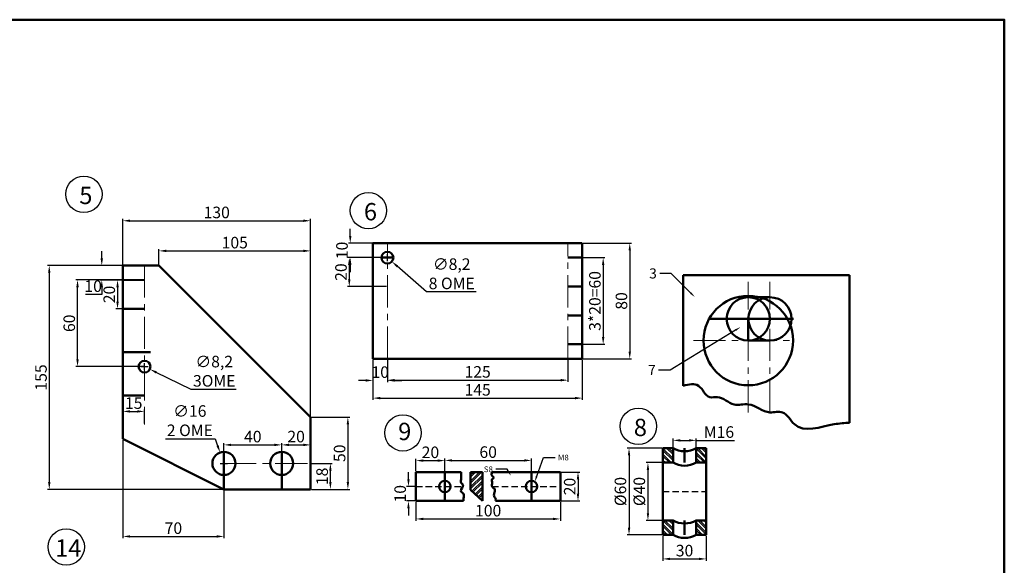
# Model space of a CAD drawing. Units: millimetres. Extents: x -749 to 333, y -22 to 680.
# Tile 4 of 4: x -349 to 333, y 302 to 680. Entities that reach past the tile are written whole.
import ezdxf
from ezdxf import colors
from ezdxf.entities.mleader import LeaderData, LeaderLine
from ezdxf.math import Vec2, Vec3

# ---------------------------------------------------------------- set-up
doc = ezdxf.new("R2010")
doc.units = ezdxf.units.MM
doc.header["$LTSCALE"] = 0.7
doc.linetypes.add('CENTER', pattern=[50.8, 31.75, -6.35, 6.35, -6.35])
doc.linetypes.add('HIDDEN', pattern=[9.525, 6.35, -3.175])
for name, color, linetype, lineweight in [('M-CNTR', 1, 'CENTER', 18), ('M-DIMS', 2, 'Continuous', 25), ('M-HATC', 8, 'Continuous', 18), ('M-HIDN', 4, 'HIDDEN', 25), ('M-OUTL', 7, 'Continuous', 50), ('M-TEXT', 3, 'Continuous', 25), ('M-TTLB', 7, 'Continuous', 50)]:
    doc.layers.add(name, color=color, linetype=linetype, lineweight=lineweight)
doc.styles.get("Standard").update_dxf_attribs({"font": 'arial.ttf'})
doc.dimstyles.new('ISO-25', dxfattribs={"dimtxt": 8, "dimasz": 5, "dimexe": 1.25, "dimexo": 0.625, "dimtad": 1, "dimtoh": 1, "dimtxsty": 'Standard', "dimcen": 2.5, "dimadec": 0, "dimazin": 0, "dimtfac": 1, "dimtofl": 0, "dimtmove": 0, "dimatfit": 3, "dimfxl": 1, "dimarcsym": 0})

# ---------------------------------------------------------------- blocks, each defined once
blk = doc.blocks.new('*D14')
at = {"layer": 'Defpoints', "color": 0, "transparency": 16777216}
for p in [(-147.78, 404.69), (-147.78, 354.69), (-121.93, 354.69)]:
    blk.add_point(p, dxfattribs=at)
at = {"layer": 'M-DIMS', "color": 0, "lineweight": -2, "transparency": 16777216}
for p, q in [((-147.16, 404.69), (-120.68, 404.69)), ((-121.93, 399.69), (-121.93, 359.69)), ((-147.16, 354.69), (-120.68, 354.69))]:
    blk.add_line(p, q, dxfattribs=at)
at = {"layer": 'M-DIMS', "color": 0, "transparency": 16777216}
for points in [[(-122.76, 399.69), (-121.1, 399.69), (-121.93, 404.69)], [(-122.76, 359.69), (-121.1, 359.69), (-121.93, 354.69)]]:
    blk.add_solid(points, dxfattribs=at)
at = {"layer": 'M-DIMS', "color": 0, "transparency": 16777216, "insert": (-126.64, 379.69), "char_height": 8, "attachment_point": 5, "rotation": 90}
blk.add_mtext('50', dxfattribs=at)
blk = doc.blocks.new('*D15')
at = {"layer": 'Defpoints', "color": 0, "transparency": 16777216}
for p in [(-147.78, 372.69), (-134.04, 372.69), (-147.78, 354.69)]:
    blk.add_point(p, dxfattribs=at)
at = {"layer": 'M-DIMS', "color": 0, "lineweight": -2, "transparency": 16777216}
for p, q in [((-147.16, 372.69), (-132.79, 372.69)), ((-134.04, 359.69), (-134.04, 367.69)), ((-147.16, 354.69), (-132.79, 354.69))]:
    blk.add_line(p, q, dxfattribs=at)
at = {"layer": 'M-DIMS', "color": 0, "transparency": 16777216}
for points in [[(-134.88, 367.69), (-133.21, 367.69), (-134.04, 372.69)], [(-134.88, 359.69), (-133.21, 359.69), (-134.04, 354.69)]]:
    blk.add_solid(points, dxfattribs=at)
at = {"layer": 'M-DIMS', "color": 0, "transparency": 16777216, "insert": (-138.75, 363.69), "char_height": 8, "attachment_point": 5, "rotation": 90}
blk.add_mtext('18', dxfattribs=at)
blk = doc.blocks.new('*D16')
at = {"layer": 'Defpoints', "color": 0, "transparency": 16777216}
for p in [(-147.78, 385.5), (-167.78, 372.69), (-147.78, 372.69)]:
    blk.add_point(p, dxfattribs=at)
at = {"layer": 'M-DIMS', "color": 0, "lineweight": -2, "transparency": 16777216}
for p, q in [((-167.78, 373.32), (-167.78, 386.75)), ((-162.78, 385.5), (-152.78, 385.5)), ((-147.78, 373.32), (-147.78, 386.75))]:
    blk.add_line(p, q, dxfattribs=at)
at = {"layer": 'M-DIMS', "color": 0, "transparency": 16777216}
for points in [[(-162.78, 386.33), (-162.78, 384.66), (-167.78, 385.5)], [(-152.78, 386.33), (-152.78, 384.66), (-147.78, 385.5)]]:
    blk.add_solid(points, dxfattribs=at)
at = {"layer": 'M-DIMS', "color": 0, "transparency": 16777216, "insert": (-157.78, 390.21), "char_height": 8, "attachment_point": 5}
blk.add_mtext('20', dxfattribs=at)
blk = doc.blocks.new('*D17')
at = {"layer": 'Defpoints', "color": 0, "transparency": 16777216}
for p in [(-167.78, 385.5), (-207.78, 372.69), (-167.78, 372.69)]:
    blk.add_point(p, dxfattribs=at)
at = {"layer": 'M-DIMS', "color": 0, "lineweight": -2, "transparency": 16777216}
for p, q in [((-207.78, 373.32), (-207.78, 386.75)), ((-202.78, 385.5), (-172.78, 385.5)), ((-167.78, 373.32), (-167.78, 386.75))]:
    blk.add_line(p, q, dxfattribs=at)
at = {"layer": 'M-DIMS', "color": 0, "transparency": 16777216}
for points in [[(-202.78, 386.33), (-202.78, 384.66), (-207.78, 385.5)], [(-172.78, 386.33), (-172.78, 384.66), (-167.78, 385.5)]]:
    blk.add_solid(points, dxfattribs=at)
at = {"layer": 'M-DIMS', "color": 0, "transparency": 16777216, "insert": (-187.78, 390.21), "char_height": 8, "attachment_point": 5}
blk.add_mtext('40', dxfattribs=at)
blk = doc.blocks.new('*D18')
at = {"layer": 'Defpoints', "color": 0, "transparency": 16777216}
for p in [(-277.78, 389.69), (-207.78, 354.69), (-207.78, 322.1)]:
    blk.add_point(p, dxfattribs=at)
at = {"layer": 'M-DIMS', "color": 0, "lineweight": -2, "transparency": 16777216}
for p, q in [((-277.78, 389.07), (-277.78, 320.85)), ((-207.78, 354.07), (-207.78, 320.85)), ((-272.78, 322.1), (-212.78, 322.1))]:
    blk.add_line(p, q, dxfattribs=at)
at = {"layer": 'M-DIMS', "color": 0, "transparency": 16777216}
for points in [[(-272.78, 322.93), (-272.78, 321.27), (-277.78, 322.1)], [(-212.78, 322.93), (-212.78, 321.27), (-207.78, 322.1)]]:
    blk.add_solid(points, dxfattribs=at)
at = {"layer": 'M-DIMS', "color": 0, "transparency": 16777216, "insert": (-242.78, 326.81), "char_height": 8, "attachment_point": 5}
blk.add_mtext('70', dxfattribs=at)
blk = doc.blocks.new('*D19')
at = {"layer": 'Defpoints', "color": 0, "transparency": 16777216}
for p in [(-147.78, 519.82), (-252.78, 509.64), (-147.78, 404.64)]:
    blk.add_point(p, dxfattribs=at)
at = {"layer": 'M-DIMS', "color": 0, "lineweight": -2, "transparency": 16777216}
for p, q in [((-252.78, 510.27), (-252.78, 521.07)), ((-247.78, 519.82), (-152.78, 519.82)), ((-147.78, 405.27), (-147.78, 521.07))]:
    blk.add_line(p, q, dxfattribs=at)
at = {"layer": 'M-DIMS', "color": 0, "transparency": 16777216}
for points in [[(-247.78, 520.66), (-247.78, 518.99), (-252.78, 519.82)], [(-152.78, 520.66), (-152.78, 518.99), (-147.78, 519.82)]]:
    blk.add_solid(points, dxfattribs=at)
at = {"layer": 'M-DIMS', "color": 0, "transparency": 16777216, "insert": (-200.28, 524.53), "char_height": 8, "attachment_point": 5}
blk.add_mtext('105', dxfattribs=at)
blk = doc.blocks.new('*D20')
at = {"layer": 'Defpoints', "color": 0, "transparency": 16777216}
for p in [(-147.78, 540.69), (-277.78, 509.69), (-147.78, 404.64)]:
    blk.add_point(p, dxfattribs=at)
at = {"layer": 'M-DIMS', "color": 0, "lineweight": -2, "transparency": 16777216}
for p, q in [((-277.78, 510.32), (-277.78, 541.94)), ((-272.78, 540.69), (-152.78, 540.69)), ((-147.78, 405.27), (-147.78, 541.94))]:
    blk.add_line(p, q, dxfattribs=at)
at = {"layer": 'M-DIMS', "color": 0, "transparency": 16777216}
for points in [[(-272.78, 541.53), (-272.78, 539.86), (-277.78, 540.69)], [(-152.78, 541.53), (-152.78, 539.86), (-147.78, 540.69)]]:
    blk.add_solid(points, dxfattribs=at)
at = {"layer": 'M-DIMS', "color": 0, "transparency": 16777216, "insert": (-212.78, 545.41), "char_height": 8, "attachment_point": 5}
blk.add_mtext('130', dxfattribs=at)
blk = doc.blocks.new('*D21')
at = {"layer": 'Defpoints', "color": 0, "transparency": 16777216}
for p in [(-277.78, 509.69), (-328.77, 354.69), (-207.78, 354.69)]:
    blk.add_point(p, dxfattribs=at)
at = {"layer": 'M-DIMS', "color": 0, "lineweight": -2, "transparency": 16777216}
for p, q in [((-278.41, 509.69), (-330.02, 509.69)), ((-328.77, 504.69), (-328.77, 359.69)), ((-208.41, 354.69), (-330.02, 354.69))]:
    blk.add_line(p, q, dxfattribs=at)
at = {"layer": 'M-DIMS', "color": 0, "transparency": 16777216}
for points in [[(-329.61, 504.69), (-327.94, 504.69), (-328.77, 509.69)], [(-329.61, 359.69), (-327.94, 359.69), (-328.77, 354.69)]]:
    blk.add_solid(points, dxfattribs=at)
at = {"layer": 'M-DIMS', "color": 0, "transparency": 16777216, "insert": (-333.48, 432.19), "char_height": 8, "attachment_point": 5, "rotation": 90}
blk.add_mtext('155', dxfattribs=at)
blk = doc.blocks.new('*D22')
at = {"layer": 'Defpoints', "color": 0, "transparency": 16777216}
for p in [(-262.78, 509.66), (-292.39, 499.66), (-262.78, 499.66)]:
    blk.add_point(p, dxfattribs=at)
at = {"layer": 'M-DIMS', "color": 0, "lineweight": -2, "transparency": 16777216}
for p, q in [((-292.39, 514.66), (-292.39, 519.66)), ((-263.41, 509.66), (-293.64, 509.66)), ((-263.41, 499.66), (-293.64, 499.66)), ((-292.39, 494.66), (-292.39, 489.66)), ((-292.39, 489.66), (-303.7, 489.66))]:
    blk.add_line(p, q, dxfattribs=at)
at = {"layer": 'M-DIMS', "color": 0, "transparency": 16777216}
for points in [[(-293.23, 514.66), (-291.56, 514.66), (-292.39, 509.66)], [(-293.23, 494.66), (-291.56, 494.66), (-292.39, 499.66)]]:
    blk.add_solid(points, dxfattribs=at)
at = {"layer": 'M-DIMS', "color": 0, "transparency": 16777216, "insert": (-298.36, 494.37), "char_height": 8, "attachment_point": 5}
blk.add_mtext('10', dxfattribs=at)
blk = doc.blocks.new('*D23')
at = {"layer": 'Defpoints', "color": 0, "transparency": 16777216}
for p in [(-262.78, 499.66), (-281.48, 479.66), (-262.78, 479.66)]:
    blk.add_point(p, dxfattribs=at)
at = {"layer": 'M-DIMS', "color": 0, "lineweight": -2, "transparency": 16777216}
for p, q in [((-263.41, 499.66), (-282.73, 499.66)), ((-281.48, 494.66), (-281.48, 484.66)), ((-263.41, 479.66), (-282.73, 479.66))]:
    blk.add_line(p, q, dxfattribs=at)
at = {"layer": 'M-DIMS', "color": 0, "transparency": 16777216}
for points in [[(-282.32, 494.66), (-280.65, 494.66), (-281.48, 499.66)], [(-282.32, 484.66), (-280.65, 484.66), (-281.48, 479.66)]]:
    blk.add_solid(points, dxfattribs=at)
at = {"layer": 'M-DIMS', "color": 0, "transparency": 16777216, "insert": (-286.19, 489.66), "char_height": 8, "attachment_point": 5, "rotation": 90}
blk.add_mtext('20', dxfattribs=at)
blk = doc.blocks.new('*D24')
at = {"layer": 'Defpoints', "color": 0, "transparency": 16777216}
for p in [(-262.78, 408.68), (-277.78, 399.69), (-262.78, 399.69)]:
    blk.add_point(p, dxfattribs=at)
at = {"layer": 'M-DIMS', "color": 0, "lineweight": -2, "transparency": 16777216}
for p, q in [((-277.78, 400.32), (-277.78, 409.93)), ((-262.78, 400.32), (-262.78, 409.93)), ((-272.78, 408.68), (-267.78, 408.68))]:
    blk.add_line(p, q, dxfattribs=at)
at = {"layer": 'M-DIMS', "color": 0, "transparency": 16777216}
for points in [[(-272.78, 409.52), (-272.78, 407.85), (-277.78, 408.68)], [(-267.78, 409.52), (-267.78, 407.85), (-262.78, 408.68)]]:
    blk.add_solid(points, dxfattribs=at)
at = {"layer": 'M-DIMS', "color": 0, "transparency": 16777216, "insert": (-270.28, 413.39), "char_height": 8, "attachment_point": 5}
blk.add_mtext('15', dxfattribs=at)
blk = doc.blocks.new('*D25')
at = {"layer": 'Defpoints', "color": 0, "transparency": 16777216}
for p in [(-210.47, 380.23), (-205.1, 365.16)]:
    blk.add_point(p, dxfattribs=at)
at = {"layer": 'M-DIMS', "color": 0, "lineweight": -2, "transparency": 16777216}
for p, q in [((-248.31, 389.65), (-213.84, 389.65)), ((-213.84, 389.65), (-212.16, 384.94)), ((-207.78, 370.19), (-207.78, 375.19)), ((-210.28, 372.69), (-205.28, 372.69))]:
    blk.add_line(p, q, dxfattribs=at)
at = {"layer": 'M-DIMS', "color": 0, "transparency": 16777216}
blk.add_solid([(-211.37, 385.22), (-212.94, 384.66), (-210.47, 380.23)], dxfattribs=at)
at = {"layer": 'M-DIMS', "color": 0, "transparency": 16777216, "insert": (-231.39, 401.22), "char_height": 8, "attachment_point": 5}
blk.add_mtext('∅16\\P2 OME', dxfattribs=at)
blk = doc.blocks.new('*D26')
at = {"layer": 'Defpoints', "color": 0, "transparency": 16777216}
for p in [(-309.2, 499.69), (-277.78, 499.69), (-262.78, 439.69)]:
    blk.add_point(p, dxfattribs=at)
at = {"layer": 'M-DIMS', "color": 0, "lineweight": -2, "transparency": 16777216}
for p, q in [((-278.41, 499.69), (-310.45, 499.69)), ((-309.2, 444.69), (-309.2, 494.69)), ((-263.41, 439.69), (-310.45, 439.69))]:
    blk.add_line(p, q, dxfattribs=at)
at = {"layer": 'M-DIMS', "color": 0, "transparency": 16777216}
for points in [[(-310.03, 494.69), (-308.36, 494.69), (-309.2, 499.69)], [(-310.03, 444.69), (-308.36, 444.69), (-309.2, 439.69)]]:
    blk.add_solid(points, dxfattribs=at)
at = {"layer": 'M-DIMS', "color": 0, "transparency": 16777216, "insert": (-313.91, 469.69), "char_height": 8, "attachment_point": 5, "rotation": 90}
blk.add_mtext('60', dxfattribs=at)
blk = doc.blocks.new('*D27')
at = {"layer": 'Defpoints', "color": 0, "transparency": 16777216}
for p in [(-266.47, 441.49), (-259.1, 437.89)]:
    blk.add_point(p, dxfattribs=at)
at = {"layer": 'M-DIMS', "color": 0, "lineweight": -2, "transparency": 16777216}
for p, q in [((-265.28, 439.69), (-260.28, 439.69)), ((-262.78, 437.19), (-262.78, 442.19)), ((-230.43, 423.89), (-254.61, 435.7)), ((-199.2, 423.89), (-230.43, 423.89))]:
    blk.add_line(p, q, dxfattribs=at)
at = {"layer": 'M-DIMS', "color": 0, "transparency": 16777216}
blk.add_solid([(-254.24, 436.45), (-254.97, 434.95), (-259.1, 437.89)], dxfattribs=at)
at = {"layer": 'M-DIMS', "color": 0, "transparency": 16777216, "insert": (-214.5, 435.47), "char_height": 8, "attachment_point": 5}
blk.add_mtext('∅8,2\\P3OME', dxfattribs=at)
blk = doc.blocks.new('*D29')
at = {"layer": 'Defpoints', "color": 0, "transparency": 16777216}
for p in [(-94.53, 525.15), (-120.27, 515.15), (-94.53, 515.15)]:
    blk.add_point(p, dxfattribs=at)
at = {"layer": 'M-DIMS', "color": 0, "lineweight": -2, "transparency": 16777216}
for p, q in [((-120.27, 530.15), (-120.27, 535.15)), ((-95.15, 525.15), (-121.52, 525.15)), ((-95.15, 515.15), (-121.52, 515.15)), ((-120.27, 510.15), (-120.27, 505.15))]:
    blk.add_line(p, q, dxfattribs=at)
at = {"layer": 'M-DIMS', "color": 0, "transparency": 16777216}
for points in [[(-121.1, 530.15), (-119.44, 530.15), (-120.27, 525.15)], [(-121.1, 510.15), (-119.44, 510.15), (-120.27, 515.15)]]:
    blk.add_solid(points, dxfattribs=at)
at = {"layer": 'M-DIMS', "color": 0, "transparency": 16777216, "insert": (-124.98, 520.15), "char_height": 8, "attachment_point": 5, "rotation": 90}
blk.add_mtext('10', dxfattribs=at)
blk = doc.blocks.new('*D28')
at = {"layer": 'Defpoints', "color": 0, "transparency": 16777216}
for p in [(-94.53, 515.15), (-120.96, 495.15), (-94.53, 495.15)]:
    blk.add_point(p, dxfattribs=at)
at = {"layer": 'M-DIMS', "color": 0, "lineweight": -2, "transparency": 16777216}
for p, q in [((-95.15, 515.15), (-122.21, 515.15)), ((-120.96, 510.15), (-120.96, 500.15)), ((-95.15, 495.15), (-122.21, 495.15))]:
    blk.add_line(p, q, dxfattribs=at)
at = {"layer": 'M-DIMS', "color": 0, "transparency": 16777216}
for points in [[(-121.79, 510.15), (-120.12, 510.15), (-120.96, 515.15)], [(-121.79, 500.15), (-120.12, 500.15), (-120.96, 495.15)]]:
    blk.add_solid(points, dxfattribs=at)
at = {"layer": 'M-DIMS', "color": 0, "transparency": 16777216, "insert": (-125.67, 505.15), "char_height": 8, "attachment_point": 5, "rotation": 90}
blk.add_mtext('20', dxfattribs=at)
blk = doc.blocks.new('*D32')
at = {"layer": 'Defpoints', "color": 0, "transparency": 16777216}
for p in [(-104.53, 445.15), (-94.53, 445.15), (-94.53, 430.12)]:
    blk.add_point(p, dxfattribs=at)
at = {"layer": 'M-DIMS', "color": 0, "lineweight": -2, "transparency": 16777216}
for p, q in [((-104.53, 444.52), (-104.53, 428.87)), ((-94.53, 444.52), (-94.53, 428.87)), ((-109.53, 430.12), (-114.53, 430.12)), ((-89.53, 430.12), (-84.53, 430.12))]:
    blk.add_line(p, q, dxfattribs=at)
at = {"layer": 'M-DIMS', "color": 0, "transparency": 16777216}
for points in [[(-109.53, 430.95), (-109.53, 429.28), (-104.53, 430.12)], [(-89.53, 430.95), (-89.53, 429.28), (-94.53, 430.12)]]:
    blk.add_solid(points, dxfattribs=at)
at = {"layer": 'M-DIMS', "color": 0, "transparency": 16777216, "insert": (-99.53, 434.83), "char_height": 8, "attachment_point": 5}
blk.add_mtext('10', dxfattribs=at)
blk = doc.blocks.new('*D33')
at = {"layer": 'Defpoints', "color": 0, "transparency": 16777216}
for p in [(-94.53, 445.15), (30.47, 445.15), (30.47, 430.31)]:
    blk.add_point(p, dxfattribs=at)
at = {"layer": 'M-DIMS', "color": 0, "lineweight": -2, "transparency": 16777216}
for p, q in [((-94.53, 444.52), (-94.53, 429.06)), ((30.47, 444.52), (30.47, 429.06)), ((-89.53, 430.31), (25.47, 430.31))]:
    blk.add_line(p, q, dxfattribs=at)
at = {"layer": 'M-DIMS', "color": 0, "transparency": 16777216}
for points in [[(-89.53, 431.14), (-89.53, 429.48), (-94.53, 430.31)], [(25.47, 431.14), (25.47, 429.48), (30.47, 430.31)]]:
    blk.add_solid(points, dxfattribs=at)
at = {"layer": 'M-DIMS', "color": 0, "transparency": 16777216, "insert": (-32.03, 435.02), "char_height": 8, "attachment_point": 5}
blk.add_mtext('125', dxfattribs=at)
blk = doc.blocks.new('*D34')
at = {"layer": 'Defpoints', "color": 0, "transparency": 16777216}
for p in [(-104.53, 445.15), (40.47, 445.15), (40.47, 417.88)]:
    blk.add_point(p, dxfattribs=at)
at = {"layer": 'M-DIMS', "color": 0, "lineweight": -2, "transparency": 16777216}
for p, q in [((-104.53, 444.52), (-104.53, 416.63)), ((40.47, 444.52), (40.47, 416.63)), ((-99.53, 417.88), (35.47, 417.88))]:
    blk.add_line(p, q, dxfattribs=at)
at = {"layer": 'M-DIMS', "color": 0, "transparency": 16777216}
for points in [[(-99.53, 418.71), (-99.53, 417.05), (-104.53, 417.88)], [(35.47, 418.71), (35.47, 417.05), (40.47, 417.88)]]:
    blk.add_solid(points, dxfattribs=at)
at = {"layer": 'M-DIMS', "color": 0, "transparency": 16777216, "insert": (-32.03, 422.59), "char_height": 8, "attachment_point": 5}
blk.add_mtext('145', dxfattribs=at)
blk = doc.blocks.new('*D30')
at = {"layer": 'Defpoints', "color": 0, "transparency": 16777216}
for p in [(30.47, 515.15), (30.47, 455.15), (54.92, 455.15)]:
    blk.add_point(p, dxfattribs=at)
at = {"layer": 'M-DIMS', "color": 0, "lineweight": -2, "transparency": 16777216}
for p, q in [((31.1, 515.15), (56.17, 515.15)), ((54.92, 510.15), (54.92, 460.15)), ((31.1, 455.15), (56.17, 455.15))]:
    blk.add_line(p, q, dxfattribs=at)
at = {"layer": 'M-DIMS', "color": 0, "transparency": 16777216}
for points in [[(54.09, 510.15), (55.75, 510.15), (54.92, 515.15)], [(54.09, 460.15), (55.75, 460.15), (54.92, 455.15)]]:
    blk.add_solid(points, dxfattribs=at)
at = {"layer": 'M-DIMS', "color": 0, "transparency": 16777216, "insert": (50.21, 485.15), "char_height": 8, "attachment_point": 5, "rotation": 90}
blk.add_mtext('3*20=60', dxfattribs=at)
blk = doc.blocks.new('*D31')
at = {"layer": 'Defpoints', "color": 0, "transparency": 16777216}
for p in [(-97.61, 517.85), (-91.45, 512.44)]:
    blk.add_point(p, dxfattribs=at)
at = {"layer": 'M-DIMS', "color": 0, "lineweight": -2, "transparency": 16777216}
for p, q in [((-97.03, 515.15), (-92.03, 515.15)), ((-94.53, 512.65), (-94.53, 517.65)), ((-67.49, 491.37), (-87.69, 509.14)), ((-33.14, 491.37), (-67.49, 491.37))]:
    blk.add_line(p, q, dxfattribs=at)
at = {"layer": 'M-DIMS', "color": 0, "transparency": 16777216}
blk.add_solid([(-87.14, 509.76), (-88.24, 508.51), (-91.45, 512.44)], dxfattribs=at)
at = {"layer": 'M-DIMS', "color": 0, "transparency": 16777216, "insert": (-50, 502.95), "char_height": 8, "attachment_point": 5}
blk.add_mtext('∅8,2\\P8 OME', dxfattribs=at)
blk = doc.blocks.new('*D35')
at = {"layer": 'Defpoints', "color": 0, "transparency": 16777216}
for p in [(40.47, 525.15), (40.47, 445.15), (73.33, 445.15)]:
    blk.add_point(p, dxfattribs=at)
at = {"layer": 'M-DIMS', "color": 0, "lineweight": -2, "transparency": 16777216}
for p, q in [((41.1, 525.15), (74.58, 525.15)), ((73.33, 520.15), (73.33, 450.15)), ((41.1, 445.15), (74.58, 445.15))]:
    blk.add_line(p, q, dxfattribs=at)
at = {"layer": 'M-DIMS', "color": 0, "transparency": 16777216}
for points in [[(72.5, 520.15), (74.16, 520.15), (73.33, 525.15)], [(72.5, 450.15), (74.16, 450.15), (73.33, 445.15)]]:
    blk.add_solid(points, dxfattribs=at)
at = {"layer": 'M-DIMS', "color": 0, "transparency": 16777216, "insert": (68.62, 485.15), "char_height": 8, "attachment_point": 5, "rotation": 90}
blk.add_mtext('80', dxfattribs=at)
blk = doc.blocks.new('*D61')
at = {"layer": 'Defpoints', "color": 0, "transparency": 16777216}
for p in [(-54.74, 374.61), (-74.74, 366.67), (-54.74, 356.67)]:
    blk.add_point(p, dxfattribs=at)
at = {"layer": 'M-DIMS', "color": 0, "lineweight": -2, "transparency": 16777216}
for p, q in [((-74.74, 367.29), (-74.74, 375.86)), ((-54.74, 357.29), (-54.74, 375.86)), ((-69.74, 374.61), (-59.74, 374.61))]:
    blk.add_line(p, q, dxfattribs=at)
at = {"layer": 'M-DIMS', "color": 0, "transparency": 16777216}
for points in [[(-69.74, 375.45), (-69.74, 373.78), (-74.74, 374.61)], [(-59.74, 375.45), (-59.74, 373.78), (-54.74, 374.61)]]:
    blk.add_solid(points, dxfattribs=at)
at = {"layer": 'M-DIMS', "color": 0, "transparency": 16777216, "insert": (-64.74, 379.32), "char_height": 8, "attachment_point": 5}
blk.add_mtext('20', dxfattribs=at)
blk = doc.blocks.new('*D62')
at = {"layer": 'Defpoints', "color": 0, "transparency": 16777216}
for p in [(5.26, 374.76), (-54.74, 366.58), (5.26, 366.58)]:
    blk.add_point(p, dxfattribs=at)
at = {"layer": 'M-DIMS', "color": 0, "lineweight": -2, "transparency": 16777216}
for p, q in [((-54.74, 367.2), (-54.74, 376.01)), ((5.26, 367.2), (5.26, 376.01)), ((-49.74, 374.76), (0.26, 374.76))]:
    blk.add_line(p, q, dxfattribs=at)
at = {"layer": 'M-DIMS', "color": 0, "transparency": 16777216}
for points in [[(-49.74, 375.59), (-49.74, 373.92), (-54.74, 374.76)], [(0.26, 375.59), (0.26, 373.92), (5.26, 374.76)]]:
    blk.add_solid(points, dxfattribs=at)
at = {"layer": 'M-DIMS', "color": 0, "transparency": 16777216, "insert": (-24.74, 379.47), "char_height": 8, "attachment_point": 5}
blk.add_mtext('60', dxfattribs=at)
blk = doc.blocks.new('*D63')
at = {"layer": 'Defpoints', "color": 0, "transparency": 16777216}
for p in [(-74.74, 346.67), (25.26, 346.67), (25.26, 334.22)]:
    blk.add_point(p, dxfattribs=at)
at = {"layer": 'M-DIMS', "color": 0, "lineweight": -2, "transparency": 16777216}
for p, q in [((-74.74, 346.04), (-74.74, 332.97)), ((25.26, 346.04), (25.26, 332.97)), ((-69.74, 334.22), (20.26, 334.22))]:
    blk.add_line(p, q, dxfattribs=at)
at = {"layer": 'M-DIMS', "color": 0, "transparency": 16777216}
for points in [[(-69.74, 335.05), (-69.74, 333.38), (-74.74, 334.22)], [(20.26, 335.05), (20.26, 333.38), (25.26, 334.22)]]:
    blk.add_solid(points, dxfattribs=at)
at = {"layer": 'M-DIMS', "color": 0, "transparency": 16777216, "insert": (-24.74, 338.93), "char_height": 8, "attachment_point": 5}
blk.add_mtext('100', dxfattribs=at)
blk = doc.blocks.new('*D64')
at = {"layer": 'Defpoints', "color": 0, "transparency": 16777216}
for p in [(25.26, 366.67), (25.26, 346.67), (37.48, 346.67)]:
    blk.add_point(p, dxfattribs=at)
at = {"layer": 'M-DIMS', "color": 0, "lineweight": -2, "transparency": 16777216}
for p, q in [((25.88, 366.67), (38.73, 366.67)), ((37.48, 361.67), (37.48, 351.67)), ((25.88, 346.67), (38.73, 346.67))]:
    blk.add_line(p, q, dxfattribs=at)
at = {"layer": 'M-DIMS', "color": 0, "transparency": 16777216}
for points in [[(36.65, 361.67), (38.32, 361.67), (37.48, 366.67)], [(36.65, 351.67), (38.32, 351.67), (37.48, 346.67)]]:
    blk.add_solid(points, dxfattribs=at)
at = {"layer": 'M-DIMS', "color": 0, "transparency": 16777216, "insert": (32.77, 356.67), "char_height": 8, "attachment_point": 5, "rotation": 90}
blk.add_mtext('20', dxfattribs=at)
blk = doc.blocks.new('*D65')
at = {"layer": 'Defpoints', "color": 0, "transparency": 16777216}
for p in [(-79.96, 356.67), (-74.74, 356.67), (-74.74, 346.67)]:
    blk.add_point(p, dxfattribs=at)
at = {"layer": 'M-DIMS', "color": 0, "lineweight": -2, "transparency": 16777216}
for p, q in [((-79.96, 361.67), (-79.96, 366.67)), ((-75.37, 356.67), (-81.21, 356.67)), ((-75.37, 346.67), (-81.21, 346.67)), ((-79.96, 341.67), (-79.96, 336.67))]:
    blk.add_line(p, q, dxfattribs=at)
at = {"layer": 'M-DIMS', "color": 0, "transparency": 16777216}
for points in [[(-80.79, 361.67), (-79.13, 361.67), (-79.96, 356.67)], [(-80.79, 341.67), (-79.13, 341.67), (-79.96, 346.67)]]:
    blk.add_solid(points, dxfattribs=at)
at = {"layer": 'M-DIMS', "color": 0, "transparency": 16777216, "insert": (-84.67, 351.67), "char_height": 8, "attachment_point": 5, "rotation": 90}
blk.add_mtext('10', dxfattribs=at)
blk = doc.blocks.new('*D83')
at = {"layer": 'Defpoints', "color": 0, "transparency": 16777216}
for p in [(103.29, 383.21), (119.29, 388.63), (119.29, 383.21)]:
    blk.add_point(p, dxfattribs=at)
at = {"layer": 'M-DIMS', "color": 0, "lineweight": -2, "transparency": 16777216}
for p, q in [((103.29, 383.84), (103.29, 389.88)), ((119.29, 383.84), (119.29, 389.88)), ((108.29, 388.63), (114.29, 388.63)), ((119.29, 388.63), (145.94, 388.63))]:
    blk.add_line(p, q, dxfattribs=at)
at = {"layer": 'M-DIMS', "color": 0, "transparency": 16777216}
for points in [[(108.29, 389.46), (108.29, 387.79), (103.29, 388.63)], [(114.29, 389.46), (114.29, 387.79), (119.29, 388.63)]]:
    blk.add_solid(points, dxfattribs=at)
at = {"layer": 'M-DIMS', "color": 0, "transparency": 16777216, "insert": (135.12, 393.34), "char_height": 8, "attachment_point": 5}
blk.add_mtext('M16', dxfattribs=at)
blk = doc.blocks.new('*D84')
at = {"layer": 'Defpoints', "color": 0, "transparency": 16777216}
for p in [(96.29, 383.21), (72.84, 323.21), (96.29, 323.21)]:
    blk.add_point(p, dxfattribs=at)
at = {"layer": 'M-DIMS', "color": 0, "lineweight": -2, "transparency": 16777216}
for p, q in [((95.67, 383.21), (71.59, 383.21)), ((72.84, 378.21), (72.84, 328.21)), ((95.67, 323.21), (71.59, 323.21))]:
    blk.add_line(p, q, dxfattribs=at)
at = {"layer": 'M-DIMS', "color": 0, "transparency": 16777216}
for points in [[(72.01, 378.21), (73.68, 378.21), (72.84, 383.21)], [(72.01, 328.21), (73.68, 328.21), (72.84, 323.21)]]:
    blk.add_solid(points, dxfattribs=at)
at = {"layer": 'M-DIMS', "color": 0, "transparency": 16777216, "insert": (67.91, 353.21), "char_height": 8, "attachment_point": 5, "rotation": 90}
blk.add_mtext('%%C60', dxfattribs=at)
blk = doc.blocks.new('*D85')
at = {"layer": 'Defpoints', "color": 0, "transparency": 16777216}
for p in [(96.29, 373.21), (85.93, 333.21), (96.29, 333.21)]:
    blk.add_point(p, dxfattribs=at)
at = {"layer": 'M-DIMS', "color": 0, "lineweight": -2, "transparency": 16777216}
for p, q in [((95.67, 373.21), (84.68, 373.21)), ((85.93, 368.21), (85.93, 338.21)), ((95.67, 333.21), (84.68, 333.21))]:
    blk.add_line(p, q, dxfattribs=at)
at = {"layer": 'M-DIMS', "color": 0, "transparency": 16777216}
for points in [[(85.09, 368.21), (86.76, 368.21), (85.93, 373.21)], [(85.09, 338.21), (86.76, 338.21), (85.93, 333.21)]]:
    blk.add_solid(points, dxfattribs=at)
at = {"layer": 'M-DIMS', "color": 0, "transparency": 16777216, "insert": (80.99, 353.21), "char_height": 8, "attachment_point": 5, "rotation": 90}
blk.add_mtext('%%C40', dxfattribs=at)
blk = doc.blocks.new('*D86')
at = {"layer": 'Defpoints', "color": 0, "transparency": 16777216}
for p in [(96.29, 323.21), (126.29, 323.21), (126.29, 306.54)]:
    blk.add_point(p, dxfattribs=at)
at = {"layer": 'M-DIMS', "color": 0, "lineweight": -2, "transparency": 16777216}
for p, q in [((96.29, 322.59), (96.29, 305.29)), ((126.29, 322.59), (126.29, 305.29)), ((101.29, 306.54), (121.29, 306.54))]:
    blk.add_line(p, q, dxfattribs=at)
at = {"layer": 'M-DIMS', "color": 0, "transparency": 16777216}
for points in [[(101.29, 307.37), (101.29, 305.7), (96.29, 306.54)], [(121.29, 307.37), (121.29, 305.7), (126.29, 306.54)]]:
    blk.add_solid(points, dxfattribs=at)
at = {"layer": 'M-DIMS', "color": 0, "transparency": 16777216, "insert": (111.29, 311.25), "char_height": 8, "attachment_point": 5}
blk.add_mtext('30', dxfattribs=at)
blk = doc.blocks.new('HOLE-8')
blk.add_line((0, 4.1), (8.2, 4.1))
blk.add_circle((4.1, 4.1), 4.1)

msp = doc.modelspace()

# ---------------------------------------------------------------- hatches: boundary and pattern name
at = {"layer": 'M-HATC', "ltscale": 0.7}
h = msp.add_hatch(dxfattribs=at)
h.set_pattern_fill('ANSI32', color=256, scale=0.3, angle=90)
h.set_pattern_definition([(135, (-3499.5471, -572.7345), (-2.0205576, -2.0205576), []), (135, (-3499.5471, -571.3875), (-2.0205576, -2.0205576), [])])
h.paths.add_polyline_path([(103.292, 333.211), (96.292, 333.211), (96.292, 323.211), (103.292, 323.211)])
h.paths.add_polyline_path([(126.292, 333.211), (119.292, 333.211), (119.292, 323.211), (126.292, 323.211)])
h.paths.add_polyline_path([(103.292, 383.211), (96.292, 383.211), (96.292, 373.211), (103.292, 373.211)])
h.paths.add_polyline_path([(126.292, 383.211), (119.292, 383.211), (119.292, 373.211), (126.292, 373.211)])
h = msp.add_hatch(dxfattribs=at)
h.set_pattern_fill('ANSI32', color=256, scale=0.3)
h.set_pattern_definition([(45, (-2972.3683, -667.5758), (-2.0205576, 2.0205576), []), (45, (-2971.0212, -667.5758), (-2.0205576, 2.0205576), [])])
h.paths.add_polyline_path([(-28.747, 366.668), (-36.966, 366.668), (-36.966, 354.288), (-28.747, 346.668)])

# ---------------------------------------------------------------- linework, layer by layer
at = {"layer": 'M-CNTR'}
for p, q in [((-94.528, 445.146), (-94.528, 525.146)), ((30.472, 445.146), (30.472, 525.146)), ((-262.785, 509.693), (-262.785, 399.662)), ((155.45, 408.038), (155.45, 498.311)), ((170.45, 408.038), (170.45, 498.311)), ((117.386, 457.742), (187.987, 457.742)), ((-207.785, 372.693), (-147.785, 372.693))]:
    msp.add_line(p, q, dxfattribs=at)
at = {"layer": 'M-HIDN'}
for p, q in [((-74.741, 356.668), (-42.306, 356.668)), ((-21.992, 356.668), (25.259, 356.668)), ((96.292, 353.211), (126.292, 353.211))]:
    msp.add_line(p, q, dxfattribs=at)
at = {"layer": 'M-OUTL'}
for p, q in [((-104.528, 525.146), (40.472, 525.146)), ((-104.528, 445.146), (-104.528, 525.146)), ((40.472, 445.146), (40.472, 525.146)), ((30.472, 515.146), (40.472, 515.146)), ((-277.785, 509.693), (-277.785, 389.693)), ((-277.785, 509.693), (-252.785, 509.642)), ((-252.785, 509.642), (-147.785, 404.693)), ((-277.785, 499.693), (-262.785, 499.662)), ((30.472, 495.146), (40.472, 495.146)), ((-277.785, 479.693), (-262.785, 479.662)), ((30.472, 475.146), (40.472, 475.146)), ((30.472, 455.146), (40.472, 455.146)), ((-277.785, 449.693), (-258.685, 449.693)), ((-104.528, 445.146), (40.472, 445.146)), ((-277.785, 419.693), (-262.785, 419.662)), ((-147.785, 354.693), (-147.785, 404.693)), ((-277.785, 389.693), (-207.785, 354.693)), ((96.292, 383.211), (96.292, 323.211)), ((103.292, 383.211), (96.292, 383.211)), ((103.292, 373.211), (103.292, 383.211)), ((111.292, 373.211), (111.292, 383.211)), ((126.292, 383.211), (119.292, 383.211)), ((119.292, 373.211), (119.292, 383.211)), ((126.292, 323.211), (126.292, 383.211)), ((-207.785, 354.693), (-207.785, 380.693)), ((-167.785, 354.693), (-167.785, 380.693)), ((96.292, 373.211), (103.292, 373.211)), ((119.292, 373.211), (126.292, 373.211)), ((-74.741, 366.668), (-74.741, 346.668)), ((-43.506, 366.668), (-74.741, 366.668)), ((-54.741, 366.668), (-54.741, 346.668)), ((-36.966, 366.668), (-36.966, 354.288)), ((-28.747, 366.668), (-36.966, 366.668)), ((-28.747, 366.668), (-28.747, 346.668)), ((25.259, 366.668), (-22.048, 366.668)), ((5.259, 366.668), (5.259, 346.668)), ((25.259, 346.668), (25.259, 366.668)), ((-207.785, 354.693), (-147.785, 354.693)), ((-36.966, 354.288), (-28.747, 346.668)), ((-74.741, 346.668), (-41.752, 346.668)), ((-19.554, 346.668), (25.259, 346.668)), ((96.292, 333.211), (103.292, 333.211)), ((103.292, 323.211), (103.292, 333.211)), ((111.292, 323.211), (111.292, 333.211)), ((119.292, 323.211), (119.292, 333.211)), ((119.292, 333.211), (126.292, 333.211)), ((96.292, 323.211), (103.292, 323.211)), ((119.292, 323.211), (126.292, 323.211))]:
    msp.add_line(p, q, dxfattribs=at)
at = {"layer": 'M-OUTL', "ltscale": 0.7}
for p, q in [((110.316, 503.084), (225.52, 503.084)), ((110.316, 503.084), (110.316, 426.396)), ((225.52, 503.084), (225.52, 400.851)), ((155.45, 487.742), (170.45, 487.742)), ((186.764, 472.742), (128.321, 472.742)), ((155.45, 457.742), (155.45, 473.742)), ((155.45, 457.742), (170.45, 457.742))]:
    msp.add_line(p, q, dxfattribs=at)
at = {"layer": 'M-OUTL'}
for centre, radius in [((155.45, 457.742), 31), ((155.45, 472.742), 15), ((170.45, 472.742), 15), ((-262.785, 439.693), 4.1), ((-207.785, 372.693), 8), ((-167.785, 372.693), 8), ((-54.741, 356.668), 4), ((5.259, 356.668), 4)]:
    msp.add_circle(centre, radius, dxfattribs=at)
for centre in [(111.292, 397.067), (111.292, 387.067), (111.292, 347.067), (111.292, 337.067)]:
    msp.add_arc(centre, 16, 240, 300, dxfattribs=at)
at = {"layer": 'M-OUTL', "ltscale": 0.7}
msp.add_open_spline([(110.316, 426.396), (114.243, 427.335), (122.27, 429.254), (126.262, 417.078), (136.852, 419.87), (144.183, 411.421), (157.947, 415.674), (167.42, 405.953), (180.957, 410.257), (189.336, 391.677), (209.733, 399.834), (222.108, 400.631), (225.52, 400.851)], degree=3, knots=[0, 0, 0, 0, 10.6329501, 21.7340026, 26.8685009, 39.5705442, 49.4205679, 65.3922454, 74.037505, 85.7195149, 113.400657, 123.9384529, 123.9384529, 123.9384529, 123.9384529], dxfattribs=at)
at = {"layer": 'M-OUTL'}
for points, knots in [([(-43.506, 366.668), (-43.52, 365.93), (-43.552, 364.191), (-43.269, 361.817), (-44.11, 359.127), (-40.522, 357.537), (-45.591, 353.65), (-40.849, 351.882), (-41.891, 348.924), (-41.791, 347.301), (-41.752, 346.668)], [0, 0, 0, 0, 2.2001963, 5.1810328, 7.4307229, 9.3472935, 13.8962006, 16.6810058, 19.7174071, 21.6569028, 21.6569028, 21.6569028, 21.6569028]), ([(-22.048, 366.668), (-22.361, 365.727), (-22.879, 364.166), (-20.035, 362.882), (-22.813, 361.636), (-21.548, 359.229), (-22.729, 356.495), (-19.765, 355.225), (-20.354, 352.286), (-21.196, 349.645), (-19.16, 348.386), (-19.403, 347.327), (-19.554, 346.668)], [0, 0, 0, 0, 2.593895, 4.3044595, 5.9348872, 8.3530342, 10.9785539, 13.3384137, 15.6808063, 19.1115757, 20.1998051, 21.9884759, 21.9884759, 21.9884759, 21.9884759])]:
    msp.add_open_spline(points, degree=3, knots=knots, dxfattribs=at)
at = {"layer": 'M-TEXT'}
for centre in [(-304.813, 559.019), (-107.671, 547.744), (79.306, 398.367), (-83.748, 393.797), (-317.031, 314.833)]:
    msp.add_circle(centre, 12.598, dxfattribs=at)
at = {"layer": 'M-TTLB', "ltscale": 0.7}
msp.add_lwpolyline([(-749.362, 679.91), (332.782, 679.91), (332.782, -22.287), (-749.362, -22.287)], close=True, dxfattribs=at)

# ---------------------------------------------------------------- block references
at = {"layer": 'M-OUTL'}
msp.add_blockref('HOLE-8', (-98.627, 511.045), dxfattribs=at)

# ---------------------------------------------------------------- texts
at = {"layer": 'M-TEXT', "char_height": 12, "attachment_point": 1}
for s, insert in [('5', (-307.961, 564.238)), ('6', (-110.819, 552.963)), ('8', (76.158, 403.586)), ('9', (-87.07, 400.808)), ('14', (-324.706, 320.052))]:
    msp.add_mtext_dynamic_manual_height_columns(s, width=30.10277, gutter_width=12.5, heights=[0], dxfattribs=dict(at, insert=insert))

# ---------------------------------------------------------------- dimensions: what is measured, and where the dimension line sits
at = {"layer": 'M-DIMS'}
for base, p1, p2, picture, middle in [((-147.785, 540.695), (-277.785, 509.693), (-147.785, 404.642), '*D20', (-212.785, 545.407)), ((-147.785, 519.822), (-252.785, 509.642), (-147.785, 404.642), '*D19', (-200.285, 524.532)), ((40.472, 417.878), (-104.528, 445.146), (40.472, 445.146), '*D34', (-32.028, 422.588)), ((-207.785, 322.1), (-277.785, 389.693), (-207.785, 354.693), '*D18', (-242.785, 326.81)), ((-167.785, 385.496), (-207.785, 372.693), (-167.785, 372.693), '*D17', (-187.785, 390.206)), ((-147.785, 385.496), (-167.785, 372.693), (-147.785, 372.693), '*D16', (-157.785, 390.206)), ((-54.741, 374.614), (-74.741, 366.668), (-54.741, 356.668), '*D61', (-64.741, 379.324)), ((5.259, 374.758), (-54.741, 366.579), (5.259, 366.579), '*D62', (-24.741, 379.468)), ((25.259, 334.217), (-74.741, 346.668), (25.259, 346.668), '*D63', (-24.741, 338.927)), ((126.292, 306.538), (96.292, 323.211), (126.292, 323.211), '*D86', (111.292, 311.25))]:
    dim = msp.add_linear_dim(base=base, p1=p1, p2=p2, dimstyle='ISO-25', override={"dimclrd": 0, "dimclre": 0, "dimclrt": 0}, dxfattribs=at)
    dim.commit()
    dim.dimension.update_dxf_attribs({"geometry": picture, "text_midpoint": middle})
for base, p1, p2, picture, middle in [((-120.269, 515.146), (-94.528, 525.146), (-94.528, 515.146), '*D29', (-120.269, 520.146)), ((-281.484, 479.662), (-262.785, 499.662), (-262.785, 479.662), '*D23', (-281.484, 489.662)), ((-121.928, 354.693), (-147.785, 404.693), (-147.785, 354.693), '*D14', (-121.928, 379.693)), ((-134.043, 372.693), (-147.785, 354.693), (-147.785, 372.693), '*D15', (-134.043, 363.693)), ((-79.961, 356.668), (-74.741, 346.668), (-74.741, 356.668), '*D65', (-79.961, 351.668))]:
    dim = msp.add_linear_dim(base=base, p1=p1, p2=p2, angle=90, dimstyle='ISO-25', override={"dimclrd": 0, "dimclre": 0, "dimclrt": 0}, dxfattribs=at)
    dim.commit()
    dim.dimension.update_dxf_attribs({"geometry": picture, "text_midpoint": middle, "dimtype": 160})
for base, p1, p2, picture, middle in [((-292.392, 499.662), (-262.785, 509.662), (-262.785, 499.662), '*D22', (-298.356, 494.372)), ((73.33, 445.146), (40.472, 525.146), (40.472, 445.146), '*D35', (68.62, 485.146)), ((-120.955, 495.146), (-94.528, 515.146), (-94.528, 495.146), '*D28', (-125.665, 505.146)), ((-328.772, 354.693), (-277.785, 509.693), (-207.785, 354.693), '*D21', (-333.482, 432.193)), ((-309.198, 499.693), (-262.785, 439.693), (-277.785, 499.693), '*D26', (-313.907, 469.693)), ((37.483, 346.668), (25.259, 366.668), (25.259, 346.668), '*D64', (32.773, 356.668))]:
    dim = msp.add_linear_dim(base=base, p1=p1, p2=p2, angle=90, dimstyle='ISO-25', override={"dimclrd": 0, "dimclre": 0, "dimclrt": 0}, dxfattribs=at)
    dim.commit()
    dim.dimension.update_dxf_attribs({"geometry": picture, "text_midpoint": middle})
for p1, p2, text, picture, middle in [((-97.606, 517.853), (-91.449, 512.438), '<>\\P8 OME', '*D31', (-50.002, 502.946)), ((-266.469, 441.493), (-259.101, 437.894), '<>\\P3OME', '*D27', (-214.5, 435.469)), ((-205.095, 365.159), (-210.474, 380.228), '<>\\P2 OME', '*D25', (-231.386, 401.224))]:
    dim = msp.add_diameter_dim_2p(p1=p1, p2=p2, text=text, dimstyle='ISO-25', override={"dimclrd": 0, "dimclre": 0, "dimclrt": 0}, dxfattribs=at)
    dim.commit()
    dim.dimension.update_dxf_attribs({"geometry": picture, "text_midpoint": middle})
for base, p1, p2, text, picture, middle in [((54.919, 455.146), (30.472, 515.146), (30.472, 455.146), '3*20=<>', '*D30', (50.207, 485.146)), ((72.842, 323.211), (96.292, 383.211), (96.292, 323.211), '%%C<>', '*D84', (67.909, 353.211)), ((85.926, 333.211), (96.292, 373.211), (96.292, 333.211), '%%C<>', '*D85', (80.993, 353.211))]:
    dim = msp.add_linear_dim(base=base, p1=p1, p2=p2, angle=90, text=text, dimstyle='ISO-25', override={"dimclrd": 0, "dimclre": 0, "dimclrt": 0}, dxfattribs=at)
    dim.commit()
    dim.dimension.update_dxf_attribs({"geometry": picture, "text_midpoint": middle})
for base, p1, p2, picture, middle in [((-94.528, 430.118), (-104.528, 445.146), (-94.528, 445.146), '*D32', (-99.528, 430.118)), ((30.472, 430.311), (-94.528, 445.146), (30.472, 445.146), '*D33', (-32.028, 430.311)), ((-262.785, 408.682), (-277.785, 399.693), (-262.785, 399.693), '*D24', (-270.285, 408.682))]:
    dim = msp.add_linear_dim(base=base, p1=p1, p2=p2, dimstyle='ISO-25', override={"dimclrd": 0, "dimclre": 0, "dimclrt": 0}, dxfattribs=at)
    dim.commit()
    dim.dimension.update_dxf_attribs({"geometry": picture, "text_midpoint": middle, "dimtype": 160})
dim = msp.add_linear_dim(base=(119.292, 388.626), p1=(103.292, 383.211), p2=(119.292, 383.211), text='M<>', dimstyle='ISO-25', override={"dimclrd": 0, "dimclre": 0, "dimclrt": 0}, dxfattribs=at)
dim.commit()
dim.dimension.update_dxf_attribs({"geometry": '*D83', "text_midpoint": (135.116, 393.336)})

# ---------------------------------------------------------------- leaders
at = {"layer": 'M-TEXT', "ltscale": 0.7}
ml = msp.add_multileader_mtext('Standard', dxfattribs=at)
ml.set_content('3', color=256)
ml.set_leader_properties()
ml.build(insert=Vec2(0, 0))
ctx = ml.context
ctx.base_point, ctx.char_height, ctx.plane_origin = Vec3(85.493, 504.162), 7, Vec3(118.401, 487.838)
ctx.text_align_type = 2
notes = []
notes.append((ctx, [(0, (1, 1, 0), (102.077, 504.162), (-1, 0), 8, [(0, [(118.401, 487.838)], 0, [])])]))
ctx.mtext.insert, ctx.mtext.alignment, ctx.mtext.flow_direction = Vec3(92.077, 507.724), 3, 5
ml = msp.add_multileader_mtext('Standard', dxfattribs=at)
ml.set_content('7', color=256)
ml.set_leader_properties()
ml.build(insert=Vec2(0, 0))
ctx = ml.context
ctx.base_point, ctx.char_height, ctx.plane_origin = Vec3(84.791, 437.33), 7, Vec3(150.047, 467.068)
ctx.text_align_type = 2
notes.append((ctx, [(0, (1, 1, 0), (101.322, 437.33), (-1, 0), 8, [(0, [(150.047, 467.068)], 0, [])])]))
ctx.mtext.insert, ctx.mtext.alignment, ctx.mtext.flow_direction = Vec3(91.322, 440.83), 3, 5
at = {"layer": 'M-TEXT'}
ml = msp.add_multileader_mtext('Standard', dxfattribs=at)
ml.set_content('M8', color=256)
ml.set_leader_properties()
ml.build(insert=Vec2(0, 0))
ctx = ml.context
ctx.base_point, ctx.plane_origin = Vec3(21.629, 376.707), Vec3(7.497, 359.983)
notes.append((ctx, [(0, (1, 1, 0), (13.629, 376.707), (1, 0), 8, [(0, [(7.497, 359.983)], 0, [])])]))
ctx.mtext.insert, ctx.mtext.flow_direction = Vec3(23.629, 378.741), 5
ml = msp.add_multileader_mtext('Standard', dxfattribs=at)
ml.set_content('S8', color=256)
ml.set_leader_properties()
ml.build(insert=Vec2(0, 0))
ctx = ml.context
ctx.base_point, ctx.plane_origin = Vec3(-29.815, 368.576), Vec3(-8.94, 363.936)
ctx.text_align_type = 2
notes.append((ctx, [(0, (1, 1, 0), (-11.477, 368.576), (-1, 0), 8, [(0, [(-8.94, 363.936)], 0, [])])]))
ctx.mtext.insert, ctx.mtext.alignment, ctx.mtext.flow_direction = Vec3(-21.477, 370.61), 3, 5
for ctx, leaders in notes:
    for number, flags, end, landing, length, lines in leaders:
        leader = LeaderData()
        leader.index, (leader.has_last_leader_line, leader.has_dogleg_vector, leader.attachment_direction) = number, flags
        leader.last_leader_point, leader.dogleg_vector, leader.dogleg_length = Vec3(end), Vec3(landing), length
        for number, points, colour, breaks in lines:
            line = LeaderLine()
            line.index, line.vertices, line.color, line.breaks = number, Vec3.list(points), colors.encode_raw_color(colour), breaks
            leader.lines.append(line)
        ctx.leaders.append(leader)

doc.saveas('drawing.dxf')
